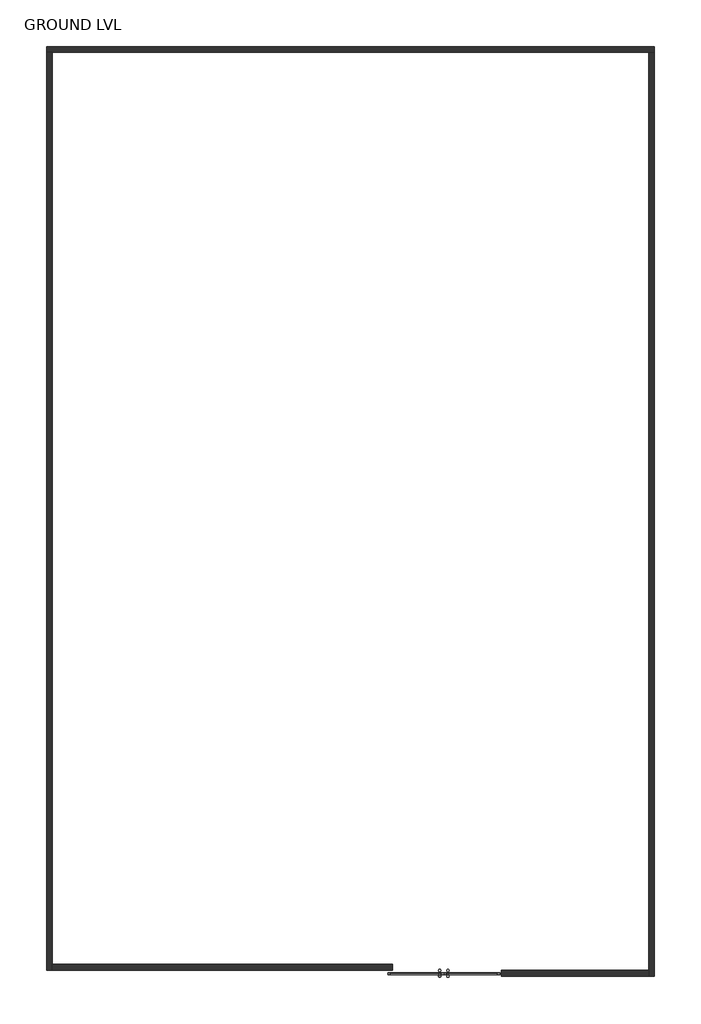
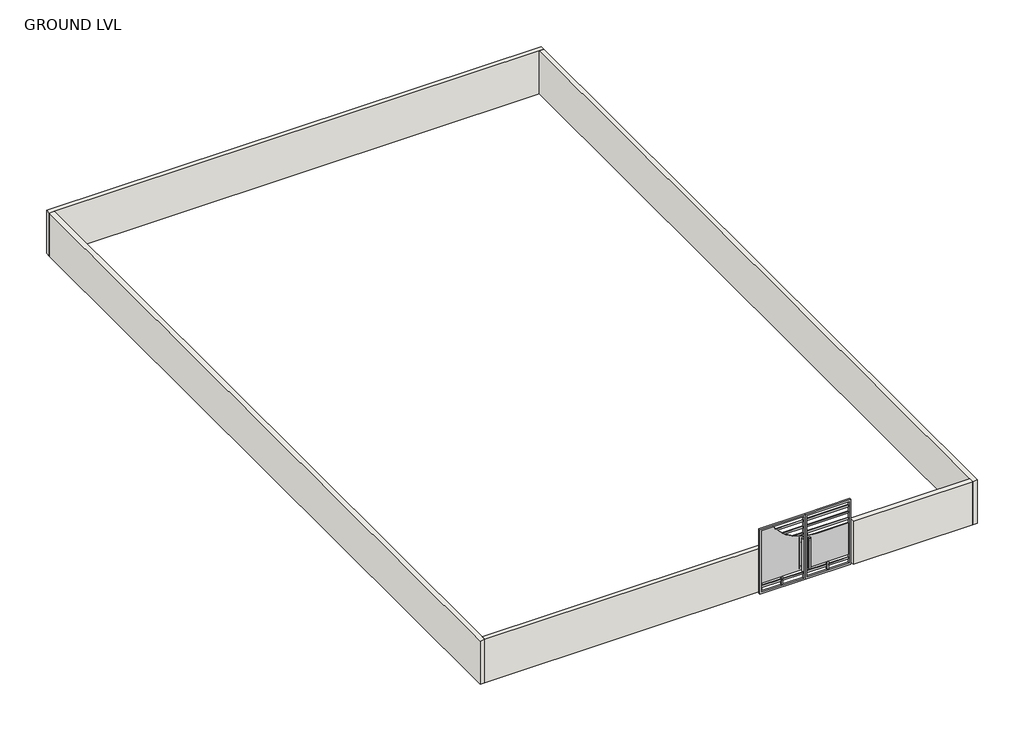
# One storey: 5 walls, 1 proxy.
"""IFC4 building model written with IfcOpenShell, lengths in millimetres."""

from ifc_helpers import new_model, si_unit, origin, origin_with_axes, place, context, project, spatial, polyline, outline, extrude, faceted_brep, transform, mapped, element, save
from components import generic_models_113f6068

model = new_model("IFC4")

# Units and contexts
model_context = context("Model", 3, world=origin())
ifc_project = project(units=[si_unit("LENGTHUNIT", "METRE", prefix="MILLI")], contexts=[model_context])

# Site, building, storey
site = spatial("IfcSite", under=ifc_project)
building = spatial("IfcBuilding", under=site)
storey = spatial("IfcBuildingStorey", under=building, Name="GROUND LVL", Elevation=0.0)

# Proxy
placement = place(None, origin())
generic_models_shape = generic_models_113f6068(model_context)
element("IfcBuildingElementProxy", 1, Name="Generic Models", at=placement, inside=storey, context=model_context, shape_type="MappedRepresentation", body=[
    mapped(generic_models_shape, transform((1573.3719693, -6031.9791112, 0.0), x_axis=(1.0, 0.0, 0.0), y_axis=(0.0, 1.0, 0.0), z_axis=(0.0, 0.0, 1.0))),
])

# Walls
element("IfcWall", 2, ObjectType="INNER WALL5\"", at=placement, inside=storey, context=model_context, shape_type="Brep", body=[
    faceted_brep([(-7074.5619351, 13983.2208888, 0.0), (-6947.5619351, 13983.2208888, 0.0), (6031.8380649, 13983.2208888, 0.0), (6158.8380649, 13983.2208888, 0.0), (6158.8380649, 13983.2208888, 1219.2), (6031.8380649, 13983.2208888, 1219.2), (-6947.5619351, 13983.2208888, 1219.2), (-7074.5619351, 13983.2208888, 1219.2), (-7074.5619351, 14110.2208888, 0.0), (-7074.5619351, 14110.2208888, 1219.2), (6158.8380649, 14110.2208888, 1219.2), (6158.8380649, 14110.2208888, 0.0)], [[[0, 1, 2, 3, 4, 5, 6, 7]], [[8, 9, 10, 11]], [[3, 2, 1, 0, 8, 11]], [[7, 6, 5, 4, 10, 9]], [[4, 3, 11, 10]], [[0, 7, 9, 8]]]),
])
element("IfcWall", 3, ObjectType="INNER WALL5\"", at=placement, inside=storey, context=model_context, shape_type="Brep", body=[
    faceted_brep([(6031.8380649, 13983.2208888, 0.0), (6031.8380649, -5981.1791112, 0.0), (6031.8380649, -6108.1791112, 0.0), (6031.8380649, -6108.1791112, 1219.2), (6031.8380649, -5981.1791112, 1219.2), (6031.8380649, 13983.2208888, 1219.2), (6158.8380649, 13983.2208888, 0.0), (6158.8380649, 13983.2208888, 1219.2), (6158.8380649, -6108.1791112, 1219.2), (6158.8380649, -6108.1791112, 0.0)], [[[0, 1, 2, 3, 4, 5]], [[6, 7, 8, 9]], [[2, 1, 0, 6, 9]], [[5, 4, 3, 8, 7]], [[0, 5, 7, 6]], [[3, 2, 9, 8]]]),
])
element("IfcWall", 4, ObjectType="INNER WALL5\"", at=placement, inside=storey, context=model_context, shape_type="SweptSolid", body=[
    extrude(outline(polyline([(2831.4380649, -5981.1791112), (6031.8380649, -5981.1791112), (6031.8380649, -6108.1791112), (2831.4380649, -6108.1791112), (2831.4380649, -5981.1791112)])), origin_with_axes(), (0.0, 0.0, 1.0), 1219.2),
])
element("IfcWall", 5, ObjectType="INNER WALL5\"", at=placement, inside=storey, context=model_context, shape_type="Brep", body=[
    faceted_brep([(-7074.5619351, 13983.2208888, 0.0), (-7074.5619351, -5981.1791112, 0.0), (-7074.5619351, -5981.1791112, 1219.2), (-7074.5619351, 13983.2208888, 1219.2), (-6947.5619351, 13983.2208888, 0.0), (-6947.5619351, 13983.2208888, 1219.2), (-6947.5619351, -5854.1791112, 1219.2), (-6947.5619351, -5981.1791112, 1219.2), (-6947.5619351, -5981.1791112, 0.0), (-6947.5619351, -5854.1791112, 0.0)], [[[0, 1, 2, 3]], [[4, 5, 6, 7, 8, 9]], [[1, 0, 4, 9, 8]], [[3, 2, 7, 6, 5]], [[0, 3, 5, 4]], [[2, 1, 8, 7]]]),
])
element("IfcWall", 6, ObjectType="INNER WALL5\"", at=placement, inside=storey, context=model_context, shape_type="SweptSolid", body=[
    extrude(outline(polyline([(456.5380649, -5981.1791112), (-6947.5619351, -5981.1791112), (-6947.5619351, -5854.1791112), (456.5380649, -5854.1791112), (456.5380649, -5981.1791112)])), origin_with_axes(), (0.0, 0.0, 1.0), 1219.2),
])

save(model, "model.ifc")

# Revit data of these elements
# Type
#   sheet = none
#   pipe = none
#   handal = none
#   faram = none
#   Default Elevation = 0
# Type "INNER WALL5\""
#   Assembly Code = "B2010"
#   Layers, outside or top first: 0' - 5" "OUTER WALL 9\"" (function 1)
# Element 1 (IfcBuildingElementProxy)
#   Phase Created = New Construction
# Elements 2, 3, 4, 5, 6 (IfcWall, "INNER WALL5\"")
#   Top Offset = 0' - 0"
#   Base Offset = 0' - 0"
#   Unconnected Height = 4' - 0"
#   wall height = 4' - 0"
#   Phase Created = New Construction
#   Base Constraint = GROUND LVL
#   Materials on its faces: "OUTER WALL 9\""
# Materials
#   "OUTER WALL 9\"": class "Generic", colour RGB 120 120 120, transparency 0, Cost = 0
